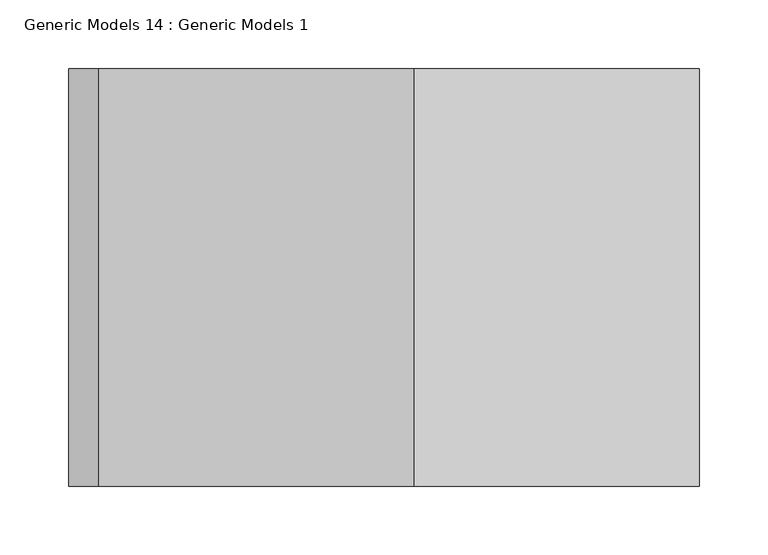
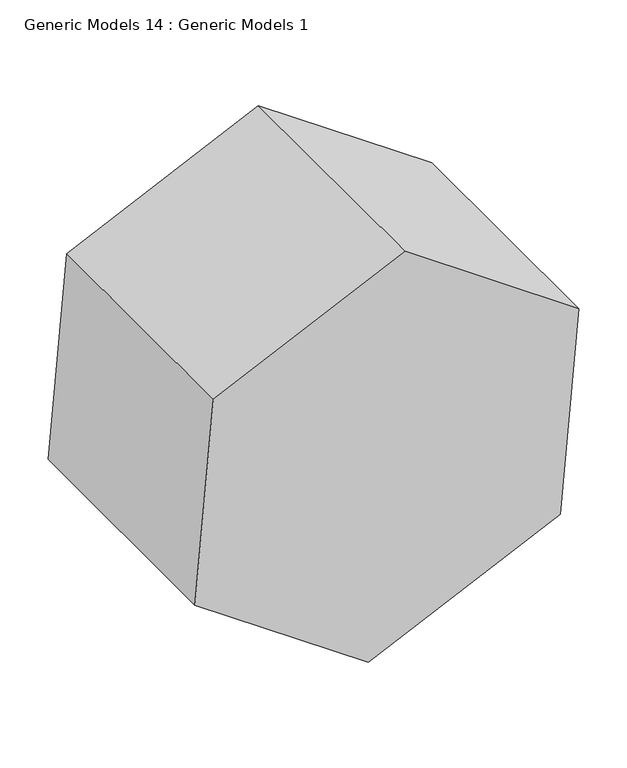
"""IFC4 building model written with IfcOpenShell, lengths in millimetres: proxy geometry, Generic Models 14 : Generic Models 1."""

from ifc_helpers import new_model, si_unit, frame, origin, place, context, project, spatial, polyline, outline, extrude, source, transform, mapped, element, save


def generic_models_14_generic_models_1_e19c2567(model_context):
    return source(origin(), model_context, "Body", "SweptSolid", [
        extrude(outline(polyline([(833.1013393, 4466.8920945), (978.7897542, 4258.8274753), (871.4447157, 4028.6252974), (618.4112624, 4006.4877387), (472.7228475, 4214.552358), (580.067886, 4444.7545359), (833.1013393, 4466.8920945)])), frame((0.0, -10720.3372434, 0.0), z_axis=(0.0, 1.0, 0.0), x_axis=(0.0, 0.0, 1.0)), (0.0, 0.0, 1.0), 304.8),
    ])


if __name__ == "__main__":
    model = new_model("IFC4")
    model_context = context("Model", 3, world=origin())
    ifc_project = project(units=[si_unit("LENGTHUNIT", "METRE", prefix="MILLI")], contexts=[model_context])
    site = spatial("IfcSite", under=ifc_project)
    building = spatial("IfcBuilding", under=site)
    placement = place(None, origin())
    generic_models_14_generic_models_1_shape = generic_models_14_generic_models_1_e19c2567(model_context)
    element("IfcBuildingElementProxy", 1, Name="Generic Models 14 : Generic Models 1", ObjectType="Generic Models 14 : Generic Models 1", at=placement, inside=building, context=model_context, shape_type="MappedRepresentation", body=[
        mapped(generic_models_14_generic_models_1_shape, transform((0.0, 0.0, 0.0), x_axis=(1.0, 0.0, 0.0), y_axis=(0.0, 1.0, 0.0), z_axis=(0.0, 0.0, 1.0))),
    ])
    save(model, "model.ifc")

# Revit data of these elements
# Element 1 (IfcBuildingElementProxy, "Generic Models 14 : Generic Models 1")
#   Materials on its faces: "Carpet (1)"
# Materials
#   "Carpet (1)": class "Carpet", colour RGB 124 80 67, transparency 0, Description = "Interior finish", Cost = 0
